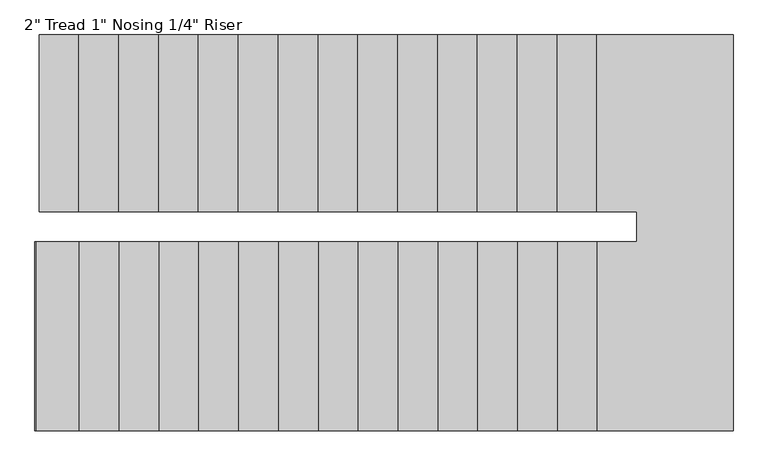
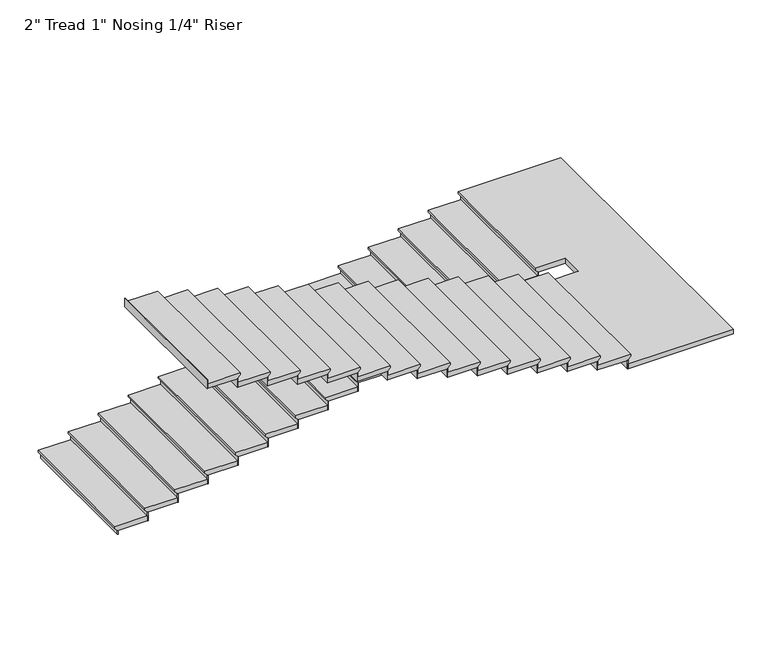
"""IFC4 building model written with IfcOpenShell, lengths in millimetres: stair flight geometry."""

from ifc_helpers import new_model, si_unit, origin, place, context, project, spatial, faceted_brep, source, transform, mapped, element, save


def stair_flight_4df775fc(model_context):
    return source(origin(), model_context, "Body", "Brep", [
        faceted_brep([(-5254.0891351, 11154.2082924, 15312.39), (-5254.0891351, 11154.2082924, 15331.44), (-5254.0891351, 12506.0715905, 15331.44), (-5254.0891351, 12506.0715905, 15312.39), (-5228.6891351, 11154.2082924, 15286.99), (-5228.6891351, 12506.0715905, 15286.99), (-4923.8891351, 11154.2082924, 15331.44), (-4923.8891351, 12506.0715905, 15331.44), (-5228.6891351, 12506.0715905, 15280.64), (-4923.8891351, 12506.0715905, 15280.64), (-4923.8891351, 11154.2082924, 15280.64), (-5228.6891351, 11154.2082924, 15280.64)], [[[0, 1, 2, 3]], [[4, 0, 3, 5]], [[2, 1, 6, 7]], [[8, 9, 10, 11]], [[2, 7, 9, 8, 5, 3]], [[8, 11, 4, 5]], [[6, 1, 0, 4, 11, 10]], [[7, 6, 10, 9]]]),
        faceted_brep([(-5228.6891351, 11154.2082924, 15280.64), (-5228.6891351, 11154.2082924, 15240.0), (-5222.3391351, 11154.2082924, 15240.0), (-5222.3391351, 11154.2082924, 15280.64), (-5228.6891351, 12506.0715905, 15280.64), (-5222.3391351, 12506.0715905, 15280.64), (-5222.3391351, 12506.0715905, 15240.0), (-5228.6891351, 12506.0715905, 15240.0)], [[[0, 1, 2, 3]], [[4, 5, 6, 7]], [[1, 0, 4, 7]], [[2, 1, 7, 6]], [[3, 2, 6, 5]], [[0, 3, 5, 4]]]),
        faceted_brep([(-4923.8891351, 11154.2082924, 15372.08), (-4923.8891351, 11154.2082924, 15280.64), (-4917.5391351, 11154.2082924, 15280.64), (-4917.5391351, 11154.2082924, 15372.08), (-4923.8891351, 12506.0715905, 15372.08), (-4917.5391351, 12506.0715905, 15372.08), (-4917.5391351, 12506.0715905, 15280.64), (-4923.8891351, 12506.0715905, 15280.64)], [[[0, 1, 2, 3]], [[4, 5, 6, 7]], [[1, 0, 4, 7]], [[2, 1, 7, 6]], [[3, 2, 6, 5]], [[0, 3, 5, 4]]]),
        faceted_brep([(-4949.2891351, 12506.0715905, 15422.88), (-4949.2891351, 11154.2082924, 15422.88), (-4619.0891351, 11154.2082924, 15422.88), (-4619.0891351, 12506.0715905, 15422.88), (-4923.8891351, 12506.0715905, 15372.08), (-4619.0891351, 12506.0715905, 15372.08), (-4619.0891351, 11154.2082924, 15372.08), (-4923.8891351, 11154.2082924, 15372.08), (-4923.8891351, 12506.0715905, 15378.43), (-4949.2891351, 12506.0715905, 15403.83), (-4923.8891351, 11154.2082924, 15378.43), (-4949.2891351, 11154.2082924, 15403.83)], [[[0, 1, 2, 3]], [[4, 5, 6, 7]], [[0, 3, 5, 4, 8, 9]], [[4, 7, 10, 8]], [[2, 1, 11, 10, 7, 6]], [[3, 2, 6, 5]], [[11, 1, 0, 9]], [[10, 11, 9, 8]]]),
        faceted_brep([(-4619.0891351, 11154.2082924, 15463.52), (-4619.0891351, 11154.2082924, 15372.08), (-4612.7391351, 11154.2082924, 15372.08), (-4612.7391351, 11154.2082924, 15463.52), (-4619.0891351, 12506.0715905, 15463.52), (-4612.7391351, 12506.0715905, 15463.52), (-4612.7391351, 12506.0715905, 15372.08), (-4619.0891351, 12506.0715905, 15372.08)], [[[0, 1, 2, 3]], [[4, 5, 6, 7]], [[1, 0, 4, 7]], [[2, 1, 7, 6]], [[3, 2, 6, 5]], [[0, 3, 5, 4]]]),
        faceted_brep([(-4644.4891351, 12506.0715905, 15514.32), (-4644.4891351, 11154.2082924, 15514.32), (-4314.2891351, 11154.2082924, 15514.32), (-4314.2891351, 12506.0715905, 15514.32), (-4619.0891351, 12506.0715905, 15463.52), (-4314.2891351, 12506.0715905, 15463.52), (-4314.2891351, 11154.2082924, 15463.52), (-4619.0891351, 11154.2082924, 15463.52), (-4619.0891351, 12506.0715905, 15469.87), (-4644.4891351, 12506.0715905, 15495.27), (-4619.0891351, 11154.2082924, 15469.87), (-4644.4891351, 11154.2082924, 15495.27)], [[[0, 1, 2, 3]], [[4, 5, 6, 7]], [[0, 3, 5, 4, 8, 9]], [[4, 7, 10, 8]], [[2, 1, 11, 10, 7, 6]], [[3, 2, 6, 5]], [[11, 1, 0, 9]], [[10, 11, 9, 8]]]),
        faceted_brep([(-4314.2891351, 11154.2082924, 15554.96), (-4314.2891351, 11154.2082924, 15463.52), (-4307.9391351, 11154.2082924, 15463.52), (-4307.9391351, 11154.2082924, 15554.96), (-4314.2891351, 12506.0715905, 15554.96), (-4307.9391351, 12506.0715905, 15554.96), (-4307.9391351, 12506.0715905, 15463.52), (-4314.2891351, 12506.0715905, 15463.52)], [[[0, 1, 2, 3]], [[4, 5, 6, 7]], [[1, 0, 4, 7]], [[2, 1, 7, 6]], [[3, 2, 6, 5]], [[0, 3, 5, 4]]]),
        faceted_brep([(-4339.6891351, 12506.0715905, 15605.76), (-4339.6891351, 11154.2082924, 15605.76), (-4009.4891351, 11154.2082924, 15605.76), (-4009.4891351, 12506.0715905, 15605.76), (-4314.2891351, 12506.0715905, 15554.96), (-4009.4891351, 12506.0715905, 15554.96), (-4009.4891351, 11154.2082924, 15554.96), (-4314.2891351, 11154.2082924, 15554.96), (-4314.2891351, 12506.0715905, 15561.31), (-4339.6891351, 12506.0715905, 15586.71), (-4314.2891351, 11154.2082924, 15561.31), (-4339.6891351, 11154.2082924, 15586.71)], [[[0, 1, 2, 3]], [[4, 5, 6, 7]], [[0, 3, 5, 4, 8, 9]], [[4, 7, 10, 8]], [[2, 1, 11, 10, 7, 6]], [[3, 2, 6, 5]], [[11, 1, 0, 9]], [[10, 11, 9, 8]]]),
        faceted_brep([(-4009.4891351, 11154.2082924, 15646.4), (-4009.4891351, 11154.2082924, 15554.96), (-4003.1391351, 11154.2082924, 15554.96), (-4003.1391351, 11154.2082924, 15646.4), (-4009.4891351, 12506.0715905, 15646.4), (-4003.1391351, 12506.0715905, 15646.4), (-4003.1391351, 12506.0715905, 15554.96), (-4009.4891351, 12506.0715905, 15554.96)], [[[0, 1, 2, 3]], [[4, 5, 6, 7]], [[1, 0, 4, 7]], [[2, 1, 7, 6]], [[3, 2, 6, 5]], [[0, 3, 5, 4]]]),
        faceted_brep([(-4034.8891351, 12506.0715905, 15697.2), (-4034.8891351, 11154.2082924, 15697.2), (-3704.6891351, 11154.2082924, 15697.2), (-3704.6891351, 12506.0715905, 15697.2), (-4009.4891351, 12506.0715905, 15646.4), (-3704.6891351, 12506.0715905, 15646.4), (-3704.6891351, 11154.2082924, 15646.4), (-4009.4891351, 11154.2082924, 15646.4), (-4009.4891351, 12506.0715905, 15652.75), (-4034.8891351, 12506.0715905, 15678.15), (-4009.4891351, 11154.2082924, 15652.75), (-4034.8891351, 11154.2082924, 15678.15)], [[[0, 1, 2, 3]], [[4, 5, 6, 7]], [[0, 3, 5, 4, 8, 9]], [[4, 7, 10, 8]], [[2, 1, 11, 10, 7, 6]], [[3, 2, 6, 5]], [[11, 1, 0, 9]], [[10, 11, 9, 8]]]),
        faceted_brep([(-3704.6891351, 11154.2082924, 15737.84), (-3704.6891351, 11154.2082924, 15646.4), (-3698.3391351, 11154.2082924, 15646.4), (-3698.3391351, 11154.2082924, 15737.84), (-3704.6891351, 12506.0715905, 15737.84), (-3698.3391351, 12506.0715905, 15737.84), (-3698.3391351, 12506.0715905, 15646.4), (-3704.6891351, 12506.0715905, 15646.4)], [[[0, 1, 2, 3]], [[4, 5, 6, 7]], [[1, 0, 4, 7]], [[2, 1, 7, 6]], [[3, 2, 6, 5]], [[0, 3, 5, 4]]]),
        faceted_brep([(-3730.0891351, 12506.0715905, 15788.64), (-3730.0891351, 11154.2082924, 15788.64), (-3399.8891351, 11154.2082924, 15788.64), (-3399.8891351, 12506.0715905, 15788.64), (-3704.6891351, 12506.0715905, 15737.84), (-3399.8891351, 12506.0715905, 15737.84), (-3399.8891351, 11154.2082924, 15737.84), (-3704.6891351, 11154.2082924, 15737.84), (-3704.6891351, 12506.0715905, 15744.19), (-3730.0891351, 12506.0715905, 15769.59), (-3704.6891351, 11154.2082924, 15744.19), (-3730.0891351, 11154.2082924, 15769.59)], [[[0, 1, 2, 3]], [[4, 5, 6, 7]], [[0, 3, 5, 4, 8, 9]], [[4, 7, 10, 8]], [[2, 1, 11, 10, 7, 6]], [[3, 2, 6, 5]], [[11, 1, 0, 9]], [[10, 11, 9, 8]]]),
        faceted_brep([(-3399.8891351, 11154.2082924, 15829.28), (-3399.8891351, 11154.2082924, 15737.84), (-3393.5391351, 11154.2082924, 15737.84), (-3393.5391351, 11154.2082924, 15829.28), (-3399.8891351, 12506.0715905, 15829.28), (-3393.5391351, 12506.0715905, 15829.28), (-3393.5391351, 12506.0715905, 15737.84), (-3399.8891351, 12506.0715905, 15737.84)], [[[0, 1, 2, 3]], [[4, 5, 6, 7]], [[1, 0, 4, 7]], [[2, 1, 7, 6]], [[3, 2, 6, 5]], [[0, 3, 5, 4]]]),
        faceted_brep([(-3425.2891351, 12506.0715905, 15880.08), (-3425.2891351, 11154.2082924, 15880.08), (-3095.0891351, 11154.2082924, 15880.08), (-3095.0891351, 12506.0715905, 15880.08), (-3399.8891351, 12506.0715905, 15829.28), (-3095.0891351, 12506.0715905, 15829.28), (-3095.0891351, 11154.2082924, 15829.28), (-3399.8891351, 11154.2082924, 15829.28), (-3399.8891351, 12506.0715905, 15835.63), (-3425.2891351, 12506.0715905, 15861.03), (-3399.8891351, 11154.2082924, 15835.63), (-3425.2891351, 11154.2082924, 15861.03)], [[[0, 1, 2, 3]], [[4, 5, 6, 7]], [[0, 3, 5, 4, 8, 9]], [[4, 7, 10, 8]], [[2, 1, 11, 10, 7, 6]], [[3, 2, 6, 5]], [[11, 1, 0, 9]], [[10, 11, 9, 8]]]),
        faceted_brep([(-3095.0891351, 11154.2082924, 15920.72), (-3095.0891351, 11154.2082924, 15829.28), (-3088.7391351, 11154.2082924, 15829.28), (-3088.7391351, 11154.2082924, 15920.72), (-3095.0891351, 12506.0715905, 15920.72), (-3088.7391351, 12506.0715905, 15920.72), (-3088.7391351, 12506.0715905, 15829.28), (-3095.0891351, 12506.0715905, 15829.28)], [[[0, 1, 2, 3]], [[4, 5, 6, 7]], [[1, 0, 4, 7]], [[2, 1, 7, 6]], [[3, 2, 6, 5]], [[0, 3, 5, 4]]]),
        faceted_brep([(-3120.4891351, 12506.0715905, 15971.52), (-3120.4891351, 11154.2082924, 15971.52), (-2790.2891351, 11154.2082924, 15971.52), (-2790.2891351, 12506.0715905, 15971.52), (-3095.0891351, 12506.0715905, 15920.72), (-2790.2891351, 12506.0715905, 15920.72), (-2790.2891351, 11154.2082924, 15920.72), (-3095.0891351, 11154.2082924, 15920.72), (-3095.0891351, 12506.0715905, 15927.07), (-3120.4891351, 12506.0715905, 15952.47), (-3095.0891351, 11154.2082924, 15927.07), (-3120.4891351, 11154.2082924, 15952.47)], [[[0, 1, 2, 3]], [[4, 5, 6, 7]], [[0, 3, 5, 4, 8, 9]], [[4, 7, 10, 8]], [[2, 1, 11, 10, 7, 6]], [[3, 2, 6, 5]], [[11, 1, 0, 9]], [[10, 11, 9, 8]]]),
        faceted_brep([(-2790.2891351, 11154.2082924, 16012.16), (-2790.2891351, 11154.2082924, 15920.72), (-2783.9391351, 11154.2082924, 15920.72), (-2783.9391351, 11154.2082924, 16012.16), (-2790.2891351, 12506.0715905, 16012.16), (-2783.9391351, 12506.0715905, 16012.16), (-2783.9391351, 12506.0715905, 15920.72), (-2790.2891351, 12506.0715905, 15920.72)], [[[0, 1, 2, 3]], [[4, 5, 6, 7]], [[1, 0, 4, 7]], [[2, 1, 7, 6]], [[3, 2, 6, 5]], [[0, 3, 5, 4]]]),
        faceted_brep([(-2815.6891351, 12506.0715905, 16062.96), (-2815.6891351, 11154.2082924, 16062.96), (-2485.4891351, 11154.2082924, 16062.96), (-2485.4891351, 12506.0715905, 16062.96), (-2790.2891351, 12506.0715905, 16012.16), (-2485.4891351, 12506.0715905, 16012.16), (-2485.4891351, 11154.2082924, 16012.16), (-2790.2891351, 11154.2082924, 16012.16), (-2790.2891351, 12506.0715905, 16018.51), (-2815.6891351, 12506.0715905, 16043.91), (-2790.2891351, 11154.2082924, 16018.51), (-2815.6891351, 11154.2082924, 16043.91)], [[[0, 1, 2, 3]], [[4, 5, 6, 7]], [[0, 3, 5, 4, 8, 9]], [[4, 7, 10, 8]], [[2, 1, 11, 10, 7, 6]], [[3, 2, 6, 5]], [[11, 1, 0, 9]], [[10, 11, 9, 8]]]),
        faceted_brep([(-2485.4891351, 11154.2082924, 16103.6), (-2485.4891351, 11154.2082924, 16012.16), (-2479.1391351, 11154.2082924, 16012.16), (-2479.1391351, 11154.2082924, 16103.6), (-2485.4891351, 12506.0715905, 16103.6), (-2479.1391351, 12506.0715905, 16103.6), (-2479.1391351, 12506.0715905, 16012.16), (-2485.4891351, 12506.0715905, 16012.16)], [[[0, 1, 2, 3]], [[4, 5, 6, 7]], [[1, 0, 4, 7]], [[2, 1, 7, 6]], [[3, 2, 6, 5]], [[0, 3, 5, 4]]]),
        faceted_brep([(-2510.8891351, 12506.0715905, 16154.4), (-2510.8891351, 11154.2082924, 16154.4), (-2180.6891351, 11154.2082924, 16154.4), (-2180.6891351, 12506.0715905, 16154.4), (-2485.4891351, 12506.0715905, 16103.6), (-2180.6891351, 12506.0715905, 16103.6), (-2180.6891351, 11154.2082924, 16103.6), (-2485.4891351, 11154.2082924, 16103.6), (-2485.4891351, 12506.0715905, 16109.95), (-2510.8891351, 12506.0715905, 16135.35), (-2485.4891351, 11154.2082924, 16109.95), (-2510.8891351, 11154.2082924, 16135.35)], [[[0, 1, 2, 3]], [[4, 5, 6, 7]], [[0, 3, 5, 4, 8, 9]], [[4, 7, 10, 8]], [[2, 1, 11, 10, 7, 6]], [[3, 2, 6, 5]], [[11, 1, 0, 9]], [[10, 11, 9, 8]]]),
        faceted_brep([(-2180.6891351, 11154.2082924, 16195.04), (-2180.6891351, 11154.2082924, 16103.6), (-2174.3391351, 11154.2082924, 16103.6), (-2174.3391351, 11154.2082924, 16195.04), (-2180.6891351, 12506.0715905, 16195.04), (-2174.3391351, 12506.0715905, 16195.04), (-2174.3391351, 12506.0715905, 16103.6), (-2180.6891351, 12506.0715905, 16103.6)], [[[0, 1, 2, 3]], [[4, 5, 6, 7]], [[1, 0, 4, 7]], [[2, 1, 7, 6]], [[3, 2, 6, 5]], [[0, 3, 5, 4]]]),
        faceted_brep([(-2206.0891351, 12506.0715905, 16245.84), (-2206.0891351, 11154.2082924, 16245.84), (-1875.8891351, 11154.2082924, 16245.84), (-1875.8891351, 12506.0715905, 16245.84), (-2180.6891351, 12506.0715905, 16195.04), (-1875.8891351, 12506.0715905, 16195.04), (-1875.8891351, 11154.2082924, 16195.04), (-2180.6891351, 11154.2082924, 16195.04), (-2180.6891351, 12506.0715905, 16201.39), (-2206.0891351, 12506.0715905, 16226.79), (-2180.6891351, 11154.2082924, 16201.39), (-2206.0891351, 11154.2082924, 16226.79)], [[[0, 1, 2, 3]], [[4, 5, 6, 7]], [[0, 3, 5, 4, 8, 9]], [[4, 7, 10, 8]], [[2, 1, 11, 10, 7, 6]], [[3, 2, 6, 5]], [[11, 1, 0, 9]], [[10, 11, 9, 8]]]),
        faceted_brep([(-1875.8891351, 11154.2082924, 16286.48), (-1875.8891351, 11154.2082924, 16195.04), (-1869.5391351, 11154.2082924, 16195.04), (-1869.5391351, 11154.2082924, 16286.48), (-1875.8891351, 12506.0715905, 16286.48), (-1869.5391351, 12506.0715905, 16286.48), (-1869.5391351, 12506.0715905, 16195.04), (-1875.8891351, 12506.0715905, 16195.04)], [[[0, 1, 2, 3]], [[4, 5, 6, 7]], [[1, 0, 4, 7]], [[2, 1, 7, 6]], [[3, 2, 6, 5]], [[0, 3, 5, 4]]]),
        faceted_brep([(-1901.2891351, 12506.0715905, 16337.28), (-1901.2891351, 11154.2082924, 16337.28), (-1571.0891351, 11154.2082924, 16337.28), (-1571.0891351, 12506.0715905, 16337.28), (-1875.8891351, 12506.0715905, 16286.48), (-1571.0891351, 12506.0715905, 16286.48), (-1571.0891351, 11154.2082924, 16286.48), (-1875.8891351, 11154.2082924, 16286.48), (-1875.8891351, 12506.0715905, 16292.83), (-1901.2891351, 12506.0715905, 16318.23), (-1875.8891351, 11154.2082924, 16292.83), (-1901.2891351, 11154.2082924, 16318.23)], [[[0, 1, 2, 3]], [[4, 5, 6, 7]], [[0, 3, 5, 4, 8, 9]], [[4, 7, 10, 8]], [[2, 1, 11, 10, 7, 6]], [[3, 2, 6, 5]], [[11, 1, 0, 9]], [[10, 11, 9, 8]]]),
        faceted_brep([(-1571.0891351, 11154.2082924, 16377.92), (-1571.0891351, 11154.2082924, 16286.48), (-1564.7391351, 11154.2082924, 16286.48), (-1564.7391351, 11154.2082924, 16377.92), (-1571.0891351, 12506.0715905, 16377.92), (-1564.7391351, 12506.0715905, 16377.92), (-1564.7391351, 12506.0715905, 16286.48), (-1571.0891351, 12506.0715905, 16286.48)], [[[0, 1, 2, 3]], [[4, 5, 6, 7]], [[1, 0, 4, 7]], [[2, 1, 7, 6]], [[3, 2, 6, 5]], [[0, 3, 5, 4]]]),
        faceted_brep([(-1596.4891351, 12506.0715905, 16428.72), (-1596.4891351, 11154.2082924, 16428.72), (-1266.2891351, 11154.2082924, 16428.72), (-1266.2891351, 12506.0715905, 16428.72), (-1571.0891351, 12506.0715905, 16377.92), (-1266.2891351, 12506.0715905, 16377.92), (-1266.2891351, 11154.2082924, 16377.92), (-1571.0891351, 11154.2082924, 16377.92), (-1571.0891351, 12506.0715905, 16384.27), (-1596.4891351, 12506.0715905, 16409.67), (-1571.0891351, 11154.2082924, 16384.27), (-1596.4891351, 11154.2082924, 16409.67)], [[[0, 1, 2, 3]], [[4, 5, 6, 7]], [[0, 3, 5, 4, 8, 9]], [[4, 7, 10, 8]], [[2, 1, 11, 10, 7, 6]], [[3, 2, 6, 5]], [[11, 1, 0, 9]], [[10, 11, 9, 8]]]),
        faceted_brep([(-1266.2891351, 11154.2082924, 16469.36), (-1266.2891351, 11154.2082924, 16377.92), (-1259.9391351, 11154.2082924, 16377.92), (-1259.9391351, 11154.2082924, 16469.36), (-1266.2891351, 12506.0715905, 16469.36), (-1259.9391351, 12506.0715905, 16469.36), (-1259.9391351, 12506.0715905, 16377.92), (-1266.2891351, 12506.0715905, 16377.92)], [[[0, 1, 2, 3]], [[4, 5, 6, 7]], [[1, 0, 4, 7]], [[2, 1, 7, 6]], [[3, 2, 6, 5]], [[0, 3, 5, 4]]]),
        faceted_brep([(-1291.6891351, 12506.0715905, 16520.16), (-1291.6891351, 11154.2082924, 16520.16), (-961.4891351, 11154.2082924, 16520.16), (-961.4891351, 12506.0715905, 16520.16), (-1266.2891351, 12506.0715905, 16469.36), (-961.4891351, 12506.0715905, 16469.36), (-961.4891351, 11154.2082924, 16469.36), (-1266.2891351, 11154.2082924, 16469.36), (-1266.2891351, 12506.0715905, 16475.71), (-1291.6891351, 12506.0715905, 16501.11), (-1266.2891351, 11154.2082924, 16475.71), (-1291.6891351, 11154.2082924, 16501.11)], [[[0, 1, 2, 3]], [[4, 5, 6, 7]], [[0, 3, 5, 4, 8, 9]], [[4, 7, 10, 8]], [[2, 1, 11, 10, 7, 6]], [[3, 2, 6, 5]], [[11, 1, 0, 9]], [[10, 11, 9, 8]]]),
        faceted_brep([(-961.4891351, 11154.2082924, 16560.8), (-961.4891351, 11154.2082924, 16469.36), (-955.1391351, 11154.2082924, 16469.36), (-955.1391351, 11154.2082924, 16560.8), (-961.4891351, 12506.0715905, 16560.8), (-955.1391351, 12506.0715905, 16560.8), (-955.1391351, 12506.0715905, 16469.36), (-961.4891351, 12506.0715905, 16469.36)], [[[0, 1, 2, 3]], [[4, 5, 6, 7]], [[1, 0, 4, 7]], [[2, 1, 7, 6]], [[3, 2, 6, 5]], [[0, 3, 5, 4]]]),
        faceted_brep([(-1012.2891351, 9478.4949943, 16611.6), (54.5108649, 9478.4949943, 16611.6), (54.5108649, 12506.0715905, 16611.6), (-986.8891351, 12506.0715905, 16611.6), (-986.8891351, 11154.2082924, 16611.6), (-682.0891351, 11154.2082924, 16611.6), (-682.0891351, 10925.6082924, 16611.6), (-1012.2891351, 10925.6082924, 16611.6), (54.5108649, 9478.4949943, 16560.8), (-1012.2891351, 9478.4949943, 16560.8), (-1012.2891351, 10925.6082924, 16560.8), (-682.0891351, 10925.6082924, 16560.8), (-682.0891351, 11154.2082924, 16560.8), (-961.4891351, 11154.2082924, 16560.8), (-961.4891351, 12506.0715905, 16560.8), (54.5108649, 12506.0715905, 16560.8), (-961.4891351, 12506.0715905, 16567.15), (-986.8891351, 12506.0715905, 16592.55), (-961.4891351, 11154.2082924, 16567.15), (-986.8891351, 11154.2082924, 16592.55)], [[[0, 1, 2, 3, 4, 5, 6, 7]], [[8, 9, 10, 11, 12, 13, 14, 15]], [[1, 0, 9, 8]], [[2, 1, 8, 15]], [[3, 2, 15, 14, 16, 17]], [[14, 13, 18, 16]], [[5, 4, 19, 18, 13, 12]], [[6, 5, 12, 11]], [[7, 6, 11, 10]], [[0, 7, 10, 9]], [[19, 4, 3, 17]], [[18, 19, 17, 16]]]),
        faceted_brep([(-1012.2891351, 10925.6082924, 16652.24), (-1012.2891351, 10925.6082924, 16560.8), (-1018.6391351, 10925.6082924, 16560.8), (-1018.6391351, 10925.6082924, 16652.24), (-1012.2891351, 9478.4949943, 16652.24), (-1018.6391351, 9478.4949943, 16652.24), (-1018.6391351, 9478.4949943, 16560.8), (-1012.2891351, 9478.4949943, 16560.8)], [[[0, 1, 2, 3]], [[4, 5, 6, 7]], [[1, 0, 4, 7]], [[2, 1, 7, 6]], [[3, 2, 6, 5]], [[0, 3, 5, 4]]]),
        faceted_brep([(-986.8891351, 9478.4949943, 16703.04), (-986.8891351, 10925.6082924, 16703.04), (-1317.0891351, 10925.6082924, 16703.04), (-1317.0891351, 9478.4949943, 16703.04), (-1012.2891351, 9478.4949943, 16652.24), (-1317.0891351, 9478.4949943, 16652.24), (-1317.0891351, 10925.6082924, 16652.24), (-1012.2891351, 10925.6082924, 16652.24), (-1012.2891351, 9478.4949943, 16658.59), (-986.8891351, 9478.4949943, 16683.99), (-1012.2891351, 10925.6082924, 16658.59), (-986.8891351, 10925.6082924, 16683.99)], [[[0, 1, 2, 3]], [[4, 5, 6, 7]], [[0, 3, 5, 4, 8, 9]], [[4, 7, 10, 8]], [[2, 1, 11, 10, 7, 6]], [[3, 2, 6, 5]], [[11, 1, 0, 9]], [[10, 11, 9, 8]]]),
        faceted_brep([(-1317.0891351, 10925.6082924, 16743.68), (-1317.0891351, 10925.6082924, 16652.24), (-1323.4391351, 10925.6082924, 16652.24), (-1323.4391351, 10925.6082924, 16743.68), (-1317.0891351, 9478.4949943, 16743.68), (-1323.4391351, 9478.4949943, 16743.68), (-1323.4391351, 9478.4949943, 16652.24), (-1317.0891351, 9478.4949943, 16652.24)], [[[0, 1, 2, 3]], [[4, 5, 6, 7]], [[1, 0, 4, 7]], [[2, 1, 7, 6]], [[3, 2, 6, 5]], [[0, 3, 5, 4]]]),
        faceted_brep([(-1291.6891351, 9478.4949943, 16794.48), (-1291.6891351, 10925.6082924, 16794.48), (-1621.8891351, 10925.6082924, 16794.48), (-1621.8891351, 9478.4949943, 16794.48), (-1317.0891351, 9478.4949943, 16743.68), (-1621.8891351, 9478.4949943, 16743.68), (-1621.8891351, 10925.6082924, 16743.68), (-1317.0891351, 10925.6082924, 16743.68), (-1317.0891351, 9478.4949943, 16750.03), (-1291.6891351, 9478.4949943, 16775.43), (-1317.0891351, 10925.6082924, 16750.03), (-1291.6891351, 10925.6082924, 16775.43)], [[[0, 1, 2, 3]], [[4, 5, 6, 7]], [[0, 3, 5, 4, 8, 9]], [[4, 7, 10, 8]], [[2, 1, 11, 10, 7, 6]], [[3, 2, 6, 5]], [[11, 1, 0, 9]], [[10, 11, 9, 8]]]),
        faceted_brep([(-1621.8891351, 10925.6082924, 16835.12), (-1621.8891351, 10925.6082924, 16743.68), (-1628.2391351, 10925.6082924, 16743.68), (-1628.2391351, 10925.6082924, 16835.12), (-1621.8891351, 9478.4949943, 16835.12), (-1628.2391351, 9478.4949943, 16835.12), (-1628.2391351, 9478.4949943, 16743.68), (-1621.8891351, 9478.4949943, 16743.68)], [[[0, 1, 2, 3]], [[4, 5, 6, 7]], [[1, 0, 4, 7]], [[2, 1, 7, 6]], [[3, 2, 6, 5]], [[0, 3, 5, 4]]]),
        faceted_brep([(-1596.4891351, 9478.4949943, 16885.92), (-1596.4891351, 10925.6082924, 16885.92), (-1926.6891351, 10925.6082924, 16885.92), (-1926.6891351, 9478.4949943, 16885.92), (-1621.8891351, 9478.4949943, 16835.12), (-1926.6891351, 9478.4949943, 16835.12), (-1926.6891351, 10925.6082924, 16835.12), (-1621.8891351, 10925.6082924, 16835.12), (-1621.8891351, 9478.4949943, 16841.47), (-1596.4891351, 9478.4949943, 16866.87), (-1621.8891351, 10925.6082924, 16841.47), (-1596.4891351, 10925.6082924, 16866.87)], [[[0, 1, 2, 3]], [[4, 5, 6, 7]], [[0, 3, 5, 4, 8, 9]], [[4, 7, 10, 8]], [[2, 1, 11, 10, 7, 6]], [[3, 2, 6, 5]], [[11, 1, 0, 9]], [[10, 11, 9, 8]]]),
        faceted_brep([(-1926.6891351, 10925.6082924, 16926.56), (-1926.6891351, 10925.6082924, 16835.12), (-1933.0391351, 10925.6082924, 16835.12), (-1933.0391351, 10925.6082924, 16926.56), (-1926.6891351, 9478.4949943, 16926.56), (-1933.0391351, 9478.4949943, 16926.56), (-1933.0391351, 9478.4949943, 16835.12), (-1926.6891351, 9478.4949943, 16835.12)], [[[0, 1, 2, 3]], [[4, 5, 6, 7]], [[1, 0, 4, 7]], [[2, 1, 7, 6]], [[3, 2, 6, 5]], [[0, 3, 5, 4]]]),
        faceted_brep([(-1901.2891351, 9478.4949943, 16977.36), (-1901.2891351, 10925.6082924, 16977.36), (-2231.4891351, 10925.6082924, 16977.36), (-2231.4891351, 9478.4949943, 16977.36), (-1926.6891351, 9478.4949943, 16926.56), (-2231.4891351, 9478.4949943, 16926.56), (-2231.4891351, 10925.6082924, 16926.56), (-1926.6891351, 10925.6082924, 16926.56), (-1926.6891351, 9478.4949943, 16932.91), (-1901.2891351, 9478.4949943, 16958.31), (-1926.6891351, 10925.6082924, 16932.91), (-1901.2891351, 10925.6082924, 16958.31)], [[[0, 1, 2, 3]], [[4, 5, 6, 7]], [[0, 3, 5, 4, 8, 9]], [[4, 7, 10, 8]], [[2, 1, 11, 10, 7, 6]], [[3, 2, 6, 5]], [[11, 1, 0, 9]], [[10, 11, 9, 8]]]),
        faceted_brep([(-2231.4891351, 10925.6082924, 17018.0), (-2231.4891351, 10925.6082924, 16926.56), (-2237.8391351, 10925.6082924, 16926.56), (-2237.8391351, 10925.6082924, 17018.0), (-2231.4891351, 9478.4949943, 17018.0), (-2237.8391351, 9478.4949943, 17018.0), (-2237.8391351, 9478.4949943, 16926.56), (-2231.4891351, 9478.4949943, 16926.56)], [[[0, 1, 2, 3]], [[4, 5, 6, 7]], [[1, 0, 4, 7]], [[2, 1, 7, 6]], [[3, 2, 6, 5]], [[0, 3, 5, 4]]]),
        faceted_brep([(-2206.0891351, 9478.4949943, 17068.8), (-2206.0891351, 10925.6082924, 17068.8), (-2536.2891351, 10925.6082924, 17068.8), (-2536.2891351, 9478.4949943, 17068.8), (-2231.4891351, 9478.4949943, 17018.0), (-2536.2891351, 9478.4949943, 17018.0), (-2536.2891351, 10925.6082924, 17018.0), (-2231.4891351, 10925.6082924, 17018.0), (-2231.4891351, 9478.4949943, 17024.35), (-2206.0891351, 9478.4949943, 17049.75), (-2231.4891351, 10925.6082924, 17024.35), (-2206.0891351, 10925.6082924, 17049.75)], [[[0, 1, 2, 3]], [[4, 5, 6, 7]], [[0, 3, 5, 4, 8, 9]], [[4, 7, 10, 8]], [[2, 1, 11, 10, 7, 6]], [[3, 2, 6, 5]], [[11, 1, 0, 9]], [[10, 11, 9, 8]]]),
        faceted_brep([(-2536.2891351, 10925.6082924, 17109.44), (-2536.2891351, 10925.6082924, 17018.0), (-2542.6391351, 10925.6082924, 17018.0), (-2542.6391351, 10925.6082924, 17109.44), (-2536.2891351, 9478.4949943, 17109.44), (-2542.6391351, 9478.4949943, 17109.44), (-2542.6391351, 9478.4949943, 17018.0), (-2536.2891351, 9478.4949943, 17018.0)], [[[0, 1, 2, 3]], [[4, 5, 6, 7]], [[1, 0, 4, 7]], [[2, 1, 7, 6]], [[3, 2, 6, 5]], [[0, 3, 5, 4]]]),
        faceted_brep([(-2510.8891351, 9478.4949943, 17160.24), (-2510.8891351, 10925.6082924, 17160.24), (-2841.0891351, 10925.6082924, 17160.24), (-2841.0891351, 9478.4949943, 17160.24), (-2536.2891351, 9478.4949943, 17109.44), (-2841.0891351, 9478.4949943, 17109.44), (-2841.0891351, 10925.6082924, 17109.44), (-2536.2891351, 10925.6082924, 17109.44), (-2536.2891351, 9478.4949943, 17115.79), (-2510.8891351, 9478.4949943, 17141.19), (-2536.2891351, 10925.6082924, 17115.79), (-2510.8891351, 10925.6082924, 17141.19)], [[[0, 1, 2, 3]], [[4, 5, 6, 7]], [[0, 3, 5, 4, 8, 9]], [[4, 7, 10, 8]], [[2, 1, 11, 10, 7, 6]], [[3, 2, 6, 5]], [[11, 1, 0, 9]], [[10, 11, 9, 8]]]),
        faceted_brep([(-2841.0891351, 10925.6082924, 17200.88), (-2841.0891351, 10925.6082924, 17109.44), (-2847.4391351, 10925.6082924, 17109.44), (-2847.4391351, 10925.6082924, 17200.88), (-2841.0891351, 9478.4949943, 17200.88), (-2847.4391351, 9478.4949943, 17200.88), (-2847.4391351, 9478.4949943, 17109.44), (-2841.0891351, 9478.4949943, 17109.44)], [[[0, 1, 2, 3]], [[4, 5, 6, 7]], [[1, 0, 4, 7]], [[2, 1, 7, 6]], [[3, 2, 6, 5]], [[0, 3, 5, 4]]]),
        faceted_brep([(-2815.6891351, 9478.4949943, 17251.68), (-2815.6891351, 10925.6082924, 17251.68), (-3145.8891351, 10925.6082924, 17251.68), (-3145.8891351, 9478.4949943, 17251.68), (-2841.0891351, 9478.4949943, 17200.88), (-3145.8891351, 9478.4949943, 17200.88), (-3145.8891351, 10925.6082924, 17200.88), (-2841.0891351, 10925.6082924, 17200.88), (-2841.0891351, 9478.4949943, 17207.23), (-2815.6891351, 9478.4949943, 17232.63), (-2841.0891351, 10925.6082924, 17207.23), (-2815.6891351, 10925.6082924, 17232.63)], [[[0, 1, 2, 3]], [[4, 5, 6, 7]], [[0, 3, 5, 4, 8, 9]], [[4, 7, 10, 8]], [[2, 1, 11, 10, 7, 6]], [[3, 2, 6, 5]], [[11, 1, 0, 9]], [[10, 11, 9, 8]]]),
        faceted_brep([(-3145.8891351, 10925.6082924, 17292.32), (-3145.8891351, 10925.6082924, 17200.88), (-3152.2391351, 10925.6082924, 17200.88), (-3152.2391351, 10925.6082924, 17292.32), (-3145.8891351, 9478.4949943, 17292.32), (-3152.2391351, 9478.4949943, 17292.32), (-3152.2391351, 9478.4949943, 17200.88), (-3145.8891351, 9478.4949943, 17200.88)], [[[0, 1, 2, 3]], [[4, 5, 6, 7]], [[1, 0, 4, 7]], [[2, 1, 7, 6]], [[3, 2, 6, 5]], [[0, 3, 5, 4]]]),
        faceted_brep([(-3120.4891351, 9478.4949943, 17343.12), (-3120.4891351, 10925.6082924, 17343.12), (-3450.6891351, 10925.6082924, 17343.12), (-3450.6891351, 9478.4949943, 17343.12), (-3145.8891351, 9478.4949943, 17292.32), (-3450.6891351, 9478.4949943, 17292.32), (-3450.6891351, 10925.6082924, 17292.32), (-3145.8891351, 10925.6082924, 17292.32), (-3145.8891351, 9478.4949943, 17298.67), (-3120.4891351, 9478.4949943, 17324.07), (-3145.8891351, 10925.6082924, 17298.67), (-3120.4891351, 10925.6082924, 17324.07)], [[[0, 1, 2, 3]], [[4, 5, 6, 7]], [[0, 3, 5, 4, 8, 9]], [[4, 7, 10, 8]], [[2, 1, 11, 10, 7, 6]], [[3, 2, 6, 5]], [[11, 1, 0, 9]], [[10, 11, 9, 8]]]),
        faceted_brep([(-3450.6891351, 10925.6082924, 17383.76), (-3450.6891351, 10925.6082924, 17292.32), (-3457.0391351, 10925.6082924, 17292.32), (-3457.0391351, 10925.6082924, 17383.76), (-3450.6891351, 9478.4949943, 17383.76), (-3457.0391351, 9478.4949943, 17383.76), (-3457.0391351, 9478.4949943, 17292.32), (-3450.6891351, 9478.4949943, 17292.32)], [[[0, 1, 2, 3]], [[4, 5, 6, 7]], [[1, 0, 4, 7]], [[2, 1, 7, 6]], [[3, 2, 6, 5]], [[0, 3, 5, 4]]]),
        faceted_brep([(-3425.2891351, 9478.4949943, 17434.56), (-3425.2891351, 10925.6082924, 17434.56), (-3755.4891351, 10925.6082924, 17434.56), (-3755.4891351, 9478.4949943, 17434.56), (-3450.6891351, 9478.4949943, 17383.76), (-3755.4891351, 9478.4949943, 17383.76), (-3755.4891351, 10925.6082924, 17383.76), (-3450.6891351, 10925.6082924, 17383.76), (-3450.6891351, 9478.4949943, 17390.11), (-3425.2891351, 9478.4949943, 17415.51), (-3450.6891351, 10925.6082924, 17390.11), (-3425.2891351, 10925.6082924, 17415.51)], [[[0, 1, 2, 3]], [[4, 5, 6, 7]], [[0, 3, 5, 4, 8, 9]], [[4, 7, 10, 8]], [[2, 1, 11, 10, 7, 6]], [[3, 2, 6, 5]], [[11, 1, 0, 9]], [[10, 11, 9, 8]]]),
        faceted_brep([(-3755.4891351, 10925.6082924, 17475.2), (-3755.4891351, 10925.6082924, 17383.76), (-3761.8391351, 10925.6082924, 17383.76), (-3761.8391351, 10925.6082924, 17475.2), (-3755.4891351, 9478.4949943, 17475.2), (-3761.8391351, 9478.4949943, 17475.2), (-3761.8391351, 9478.4949943, 17383.76), (-3755.4891351, 9478.4949943, 17383.76)], [[[0, 1, 2, 3]], [[4, 5, 6, 7]], [[1, 0, 4, 7]], [[2, 1, 7, 6]], [[3, 2, 6, 5]], [[0, 3, 5, 4]]]),
        faceted_brep([(-3730.0891351, 9478.4949943, 17526.0), (-3730.0891351, 10925.6082924, 17526.0), (-4060.2891351, 10925.6082924, 17526.0), (-4060.2891351, 9478.4949943, 17526.0), (-3755.4891351, 9478.4949943, 17475.2), (-4060.2891351, 9478.4949943, 17475.2), (-4060.2891351, 10925.6082924, 17475.2), (-3755.4891351, 10925.6082924, 17475.2), (-3755.4891351, 9478.4949943, 17481.55), (-3730.0891351, 9478.4949943, 17506.95), (-3755.4891351, 10925.6082924, 17481.55), (-3730.0891351, 10925.6082924, 17506.95)], [[[0, 1, 2, 3]], [[4, 5, 6, 7]], [[0, 3, 5, 4, 8, 9]], [[4, 7, 10, 8]], [[2, 1, 11, 10, 7, 6]], [[3, 2, 6, 5]], [[11, 1, 0, 9]], [[10, 11, 9, 8]]]),
        faceted_brep([(-4060.2891351, 10925.6082924, 17566.64), (-4060.2891351, 10925.6082924, 17475.2), (-4066.6391351, 10925.6082924, 17475.2), (-4066.6391351, 10925.6082924, 17566.64), (-4060.2891351, 9478.4949943, 17566.64), (-4066.6391351, 9478.4949943, 17566.64), (-4066.6391351, 9478.4949943, 17475.2), (-4060.2891351, 9478.4949943, 17475.2)], [[[0, 1, 2, 3]], [[4, 5, 6, 7]], [[1, 0, 4, 7]], [[2, 1, 7, 6]], [[3, 2, 6, 5]], [[0, 3, 5, 4]]]),
        faceted_brep([(-4034.8891351, 9478.4949943, 17617.44), (-4034.8891351, 10925.6082924, 17617.44), (-4365.0891351, 10925.6082924, 17617.44), (-4365.0891351, 9478.4949943, 17617.44), (-4060.2891351, 9478.4949943, 17566.64), (-4365.0891351, 9478.4949943, 17566.64), (-4365.0891351, 10925.6082924, 17566.64), (-4060.2891351, 10925.6082924, 17566.64), (-4060.2891351, 9478.4949943, 17572.99), (-4034.8891351, 9478.4949943, 17598.39), (-4060.2891351, 10925.6082924, 17572.99), (-4034.8891351, 10925.6082924, 17598.39)], [[[0, 1, 2, 3]], [[4, 5, 6, 7]], [[0, 3, 5, 4, 8, 9]], [[4, 7, 10, 8]], [[2, 1, 11, 10, 7, 6]], [[3, 2, 6, 5]], [[11, 1, 0, 9]], [[10, 11, 9, 8]]]),
        faceted_brep([(-4365.0891351, 10925.6082924, 17658.08), (-4365.0891351, 10925.6082924, 17566.64), (-4371.4391351, 10925.6082924, 17566.64), (-4371.4391351, 10925.6082924, 17658.08), (-4365.0891351, 9478.4949943, 17658.08), (-4371.4391351, 9478.4949943, 17658.08), (-4371.4391351, 9478.4949943, 17566.64), (-4365.0891351, 9478.4949943, 17566.64)], [[[0, 1, 2, 3]], [[4, 5, 6, 7]], [[1, 0, 4, 7]], [[2, 1, 7, 6]], [[3, 2, 6, 5]], [[0, 3, 5, 4]]]),
        faceted_brep([(-4339.6891351, 9478.4949943, 17708.88), (-4339.6891351, 10925.6082924, 17708.88), (-4669.8891351, 10925.6082924, 17708.88), (-4669.8891351, 9478.4949943, 17708.88), (-4365.0891351, 9478.4949943, 17658.08), (-4669.8891351, 9478.4949943, 17658.08), (-4669.8891351, 10925.6082924, 17658.08), (-4365.0891351, 10925.6082924, 17658.08), (-4365.0891351, 9478.4949943, 17664.43), (-4339.6891351, 9478.4949943, 17689.83), (-4365.0891351, 10925.6082924, 17664.43), (-4339.6891351, 10925.6082924, 17689.83)], [[[0, 1, 2, 3]], [[4, 5, 6, 7]], [[0, 3, 5, 4, 8, 9]], [[4, 7, 10, 8]], [[2, 1, 11, 10, 7, 6]], [[3, 2, 6, 5]], [[11, 1, 0, 9]], [[10, 11, 9, 8]]]),
        faceted_brep([(-4669.8891351, 10925.6082924, 17749.52), (-4669.8891351, 10925.6082924, 17658.08), (-4676.2391351, 10925.6082924, 17658.08), (-4676.2391351, 10925.6082924, 17749.52), (-4669.8891351, 9478.4949943, 17749.52), (-4676.2391351, 9478.4949943, 17749.52), (-4676.2391351, 9478.4949943, 17658.08), (-4669.8891351, 9478.4949943, 17658.08)], [[[0, 1, 2, 3]], [[4, 5, 6, 7]], [[1, 0, 4, 7]], [[2, 1, 7, 6]], [[3, 2, 6, 5]], [[0, 3, 5, 4]]]),
        faceted_brep([(-4644.4891351, 9478.4949943, 17800.32), (-4644.4891351, 10925.6082924, 17800.32), (-4974.6891351, 10925.6082924, 17800.32), (-4974.6891351, 9478.4949943, 17800.32), (-4669.8891351, 9478.4949943, 17749.52), (-4974.6891351, 9478.4949943, 17749.52), (-4974.6891351, 10925.6082924, 17749.52), (-4669.8891351, 10925.6082924, 17749.52), (-4669.8891351, 9478.4949943, 17755.87), (-4644.4891351, 9478.4949943, 17781.27), (-4669.8891351, 10925.6082924, 17755.87), (-4644.4891351, 10925.6082924, 17781.27)], [[[0, 1, 2, 3]], [[4, 5, 6, 7]], [[0, 3, 5, 4, 8, 9]], [[4, 7, 10, 8]], [[2, 1, 11, 10, 7, 6]], [[3, 2, 6, 5]], [[11, 1, 0, 9]], [[10, 11, 9, 8]]]),
        faceted_brep([(-4974.6891351, 10925.6082924, 17840.96), (-4974.6891351, 10925.6082924, 17749.52), (-4981.0391351, 10925.6082924, 17749.52), (-4981.0391351, 10925.6082924, 17840.96), (-4974.6891351, 9478.4949943, 17840.96), (-4981.0391351, 9478.4949943, 17840.96), (-4981.0391351, 9478.4949943, 17749.52), (-4974.6891351, 9478.4949943, 17749.52)], [[[0, 1, 2, 3]], [[4, 5, 6, 7]], [[1, 0, 4, 7]], [[2, 1, 7, 6]], [[3, 2, 6, 5]], [[0, 3, 5, 4]]]),
        faceted_brep([(-5279.4891351, 10925.6082924, 17932.4), (-5279.4891351, 10925.6082924, 17840.96), (-5285.8391351, 10925.6082924, 17840.96), (-5285.8391351, 10925.6082924, 17932.4), (-5279.4891351, 9478.4949943, 17932.4), (-5285.8391351, 9478.4949943, 17932.4), (-5285.8391351, 9478.4949943, 17840.96), (-5279.4891351, 9478.4949943, 17840.96)], [[[0, 1, 2, 3]], [[4, 5, 6, 7]], [[1, 0, 4, 7]], [[2, 1, 7, 6]], [[3, 2, 6, 5]], [[0, 3, 5, 4]]]),
        faceted_brep([(-4949.2891351, 9478.4949943, 17891.76), (-4949.2891351, 10925.6082924, 17891.76), (-5279.4891351, 10925.6082924, 17891.76), (-5279.4891351, 9478.4949943, 17891.76), (-4974.6891351, 9478.4949943, 17840.96), (-5279.4891351, 9478.4949943, 17840.96), (-5279.4891351, 10925.6082924, 17840.96), (-4974.6891351, 10925.6082924, 17840.96), (-4974.6891351, 9478.4949943, 17847.31), (-4949.2891351, 9478.4949943, 17872.71), (-4974.6891351, 10925.6082924, 17847.31), (-4949.2891351, 10925.6082924, 17872.71)], [[[0, 1, 2, 3]], [[4, 5, 6, 7]], [[0, 3, 5, 4, 8, 9]], [[4, 7, 10, 8]], [[2, 1, 11, 10, 7, 6]], [[3, 2, 6, 5]], [[11, 1, 0, 9]], [[10, 11, 9, 8]]]),
    ])


if __name__ == "__main__":
    model = new_model("IFC4")
    model_context = context("Model", 3, world=origin())
    ifc_project = project(units=[si_unit("LENGTHUNIT", "METRE", prefix="MILLI")], contexts=[model_context])
    site = spatial("IfcSite", under=ifc_project)
    building = spatial("IfcBuilding", under=site)
    placement = place(None, origin())
    stair_flight_shape = stair_flight_4df775fc(model_context)
    element("IfcStairFlight", 1, ObjectType="2\" Tread 1\" Nosing 1/4\" Riser", at=placement, inside=building, context=model_context, shape_type="MappedRepresentation", body=[
        mapped(stair_flight_shape, transform((0.0, 0.0, 0.0), x_axis=(1.0, 0.0, 0.0), y_axis=(0.0, 1.0, 0.0), z_axis=(0.0, 0.0, 1.0))),
    ])
    save(model, "model.ifc")
